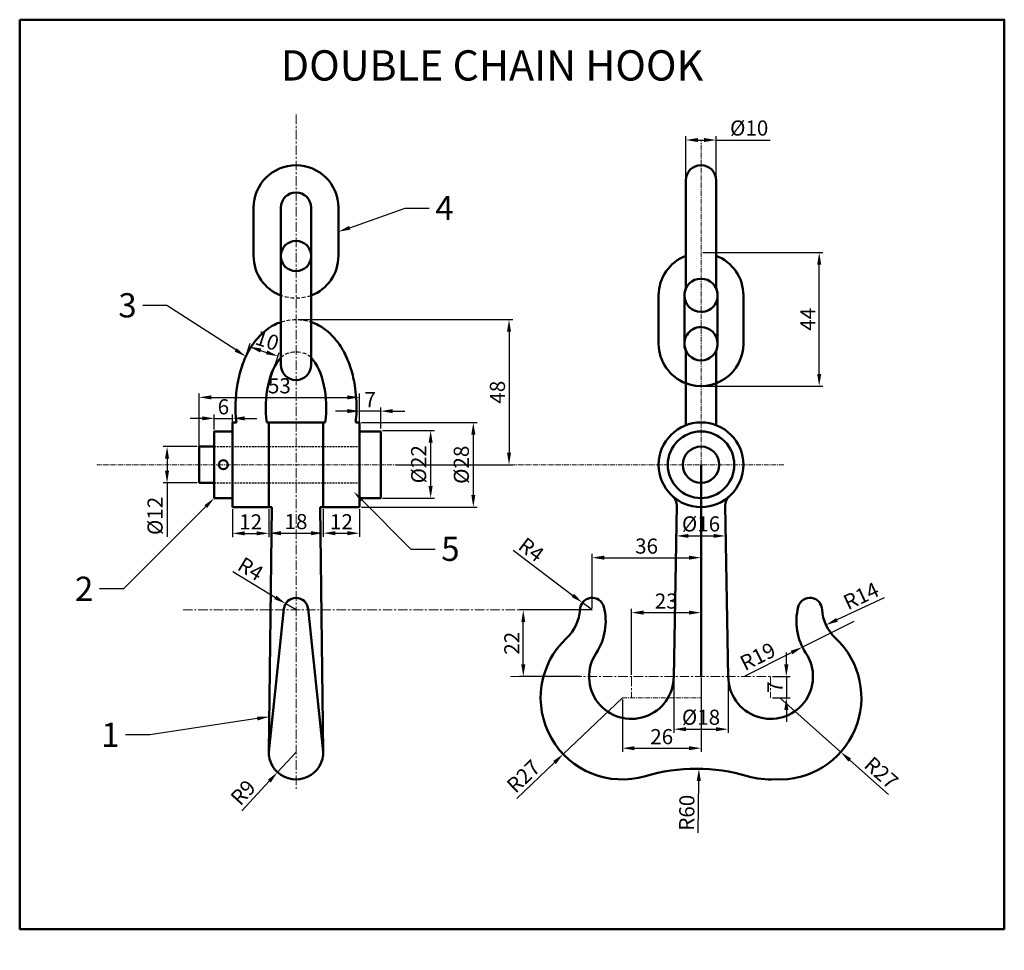
# Model space of a CAD drawing. Units: millimetres. Extents: x -60 to 265, y -36 to 271.
import ezdxf
from ezdxf import colors
from ezdxf.entities.mleader import LeaderData, LeaderLine
from ezdxf.math import Vec2, Vec3

# ---------------------------------------------------------------- set-up
doc = ezdxf.new("R2010")
doc.units = ezdxf.units.MM
doc.header["$LTSCALE"] = 0.1
doc.linetypes.add('CENTER', pattern=[50.8, 31.75, -6.35, 6.35, -6.35])
doc.linetypes.add('DASHED', pattern=[19.05, 12.7, -6.35])
for name, color, linetype, lineweight in [('M-CNTR', 1, 'CENTER', 18), ('M-DIMS', 2, 'Continuous', 25), ('M-HIDN', 4, 'DASHED', 25), ('M-OUTL', 7, 'Continuous', 50), ('M-TEXT', 3, 'Continuous', 25), ('M-TTLB', 7, 'Continuous', 50)]:
    doc.layers.add(name, color=color, linetype=linetype, lineweight=lineweight)
doc.styles.get("Standard").update_dxf_attribs({"font": 'arial.ttf'})
doc.dimstyles.new('ISO-25', dxfattribs={"dimtxt": 5, "dimasz": 4, "dimexe": 1.25, "dimexo": 0.625, "dimtad": 1, "dimdec": 0, "dimtxsty": 'Standard', "dimcen": 2.5, "dimadec": 0, "dimazin": 0, "dimtfac": 1, "dimtdec": 0, "dimtmove": 0, "dimatfit": 3, "dimfxl": 1, "dimarcsym": 0})

# ---------------------------------------------------------------- blocks, each defined once
blk = doc.blocks.new('*D1')
at = {"layer": 'Defpoints', "color": 0, "ltscale": 0.5, "transparency": 16777216}
for p in [(190.82, 47.23), (211, 29.28)]:
    blk.add_point(p, dxfattribs=at)
at = {"layer": 'M-DIMS', "color": 0, "lineweight": -2, "ltscale": 0.5, "transparency": 16777216}
for p, q in [((190.82, 47.23), (211, 29.28)), ((226.83, 15.2), (213.98, 26.63))]:
    blk.add_line(p, q, dxfattribs=at)
at = {"layer": 'M-DIMS', "color": 0, "ltscale": 0.5, "transparency": 16777216}
blk.add_solid([(214.43, 27.12), (213.54, 26.13), (211, 29.28)], dxfattribs=at)
at = {"layer": 'M-DIMS', "color": 0, "ltscale": 0.5, "transparency": 16777216, "insert": (223.99, 21.92), "char_height": 5, "attachment_point": 5, "rotation": 318.3453}
blk.add_mtext('R27', dxfattribs=at)
blk = doc.blocks.new('*D2')
at = {"layer": 'Defpoints', "color": 0, "ltscale": 0.5, "transparency": 16777216}
for p in [(164.12, 23.74), (163.32, -36.25)]:
    blk.add_point(p, dxfattribs=at)
at = {"layer": 'M-DIMS', "color": 0, "lineweight": -2, "ltscale": 0.5, "transparency": 16777216}
blk.add_line((163.84, 2.57), (164.07, 19.75), dxfattribs=at)
at = {"layer": 'M-DIMS', "color": 0, "ltscale": 0.5, "transparency": 16777216}
blk.add_solid([(163.4, 19.75), (164.74, 19.74), (164.12, 23.74)], dxfattribs=at)
at = {"layer": 'M-DIMS', "color": 0, "ltscale": 0.5, "transparency": 16777216, "insert": (160.75, 9.2), "char_height": 5, "attachment_point": 5, "rotation": 89.2359}
blk.add_mtext('R60', dxfattribs=at)
blk = doc.blocks.new('*D3')
at = {"layer": 'Defpoints', "color": 0, "ltscale": 0.5, "transparency": 16777216}
for p in [(218.8, 77.2), (206.11, 71.28)]:
    blk.add_point(p, dxfattribs=at)
at = {"layer": 'M-DIMS', "color": 0, "lineweight": -2, "ltscale": 0.5, "transparency": 16777216}
blk.add_line((225.3, 80.24), (209.74, 72.97), dxfattribs=at)
at = {"layer": 'M-DIMS', "color": 0, "ltscale": 0.5, "transparency": 16777216}
blk.add_solid([(209.45, 73.58), (210.02, 72.37), (206.11, 71.28)], dxfattribs=at)
at = {"layer": 'M-DIMS', "color": 0, "ltscale": 0.5, "transparency": 16777216, "insert": (218, 80.29), "char_height": 5, "attachment_point": 5, "rotation": 25.0408}
blk.add_mtext('R14', dxfattribs=at)
blk = doc.blocks.new('*D4')
at = {"layer": 'Defpoints', "color": 0, "ltscale": 0.5, "transparency": 16777216}
for p in [(215.34, 72.45), (198.33, 63.97)]:
    blk.add_point(p, dxfattribs=at)
at = {"layer": 'M-DIMS', "color": 0, "lineweight": -2, "ltscale": 0.5, "transparency": 16777216}
for p, q in [((215.34, 72.45), (198.33, 63.97)), ((179.36, 54.5), (194.76, 62.18))]:
    blk.add_line(p, q, dxfattribs=at)
at = {"layer": 'M-DIMS', "color": 0, "ltscale": 0.5, "transparency": 16777216}
blk.add_solid([(194.46, 62.78), (195.05, 61.59), (198.33, 63.97)], dxfattribs=at)
at = {"layer": 'M-DIMS', "color": 0, "ltscale": 0.5, "transparency": 16777216, "insert": (183.85, 60.3), "char_height": 5, "attachment_point": 5, "rotation": 26.5038}
blk.add_mtext('R19', dxfattribs=at)
blk = doc.blocks.new('*D5')
at = {"layer": 'Defpoints', "color": 0, "ltscale": 0.5, "transparency": 16777216}
for p in [(125.63, 78.64), (128.82, 76.23)]:
    blk.add_point(p, dxfattribs=at)
at = {"layer": 'M-DIMS', "color": 0, "lineweight": -2, "ltscale": 0.5, "transparency": 16777216}
for p, q in [((102.74, 95.97), (122.44, 81.06)), ((128.82, 76.23), (125.63, 78.64))]:
    blk.add_line(p, q, dxfattribs=at)
at = {"layer": 'M-DIMS', "color": 0, "ltscale": 0.5, "transparency": 16777216}
blk.add_solid([(122.85, 81.59), (122.04, 80.52), (125.63, 78.64)], dxfattribs=at)
at = {"layer": 'M-DIMS', "color": 0, "ltscale": 0.5, "transparency": 16777216, "insert": (108.33, 95.65), "char_height": 5, "attachment_point": 5, "rotation": 322.8841}
blk.add_mtext('R4', dxfattribs=at)
blk = doc.blocks.new('*D6')
at = {"layer": 'Defpoints', "color": 0, "ltscale": 0.5, "transparency": 16777216}
for p in [(164.82, 93.52), (128.82, 76.23), (164.82, 76.23)]:
    blk.add_point(p, dxfattribs=at)
at = {"layer": 'M-DIMS', "color": 0, "lineweight": -2, "ltscale": 0.5, "transparency": 16777216}
for p, q in [((128.82, 76.85), (128.82, 94.77)), ((164.82, 76.85), (164.82, 94.77)), ((132.82, 93.52), (160.82, 93.52))]:
    blk.add_line(p, q, dxfattribs=at)
at = {"layer": 'M-DIMS', "color": 0, "ltscale": 0.5, "transparency": 16777216}
for points in [[(132.82, 94.19), (132.82, 92.86), (128.82, 93.52)], [(160.82, 94.19), (160.82, 92.86), (164.82, 93.52)]]:
    blk.add_solid(points, dxfattribs=at)
at = {"layer": 'M-DIMS', "color": 0, "ltscale": 0.5, "transparency": 16777216, "insert": (146.82, 96.7), "char_height": 5, "attachment_point": 5}
blk.add_mtext('36', dxfattribs=at)
blk = doc.blocks.new('*D7')
at = {"layer": 'Defpoints', "color": 0, "ltscale": 0.5, "transparency": 16777216}
for p in [(106.08, 76.23), (128.82, 76.23), (125.49, 54.23)]:
    blk.add_point(p, dxfattribs=at)
at = {"layer": 'M-DIMS', "color": 0, "lineweight": -2, "ltscale": 0.5, "transparency": 16777216}
for p, q in [((128.2, 76.23), (104.83, 76.23)), ((106.08, 58.23), (106.08, 72.23)), ((124.87, 54.23), (104.83, 54.23))]:
    blk.add_line(p, q, dxfattribs=at)
at = {"layer": 'M-DIMS', "color": 0, "ltscale": 0.5, "transparency": 16777216}
for points in [[(105.41, 72.23), (106.74, 72.23), (106.08, 76.23)], [(105.41, 58.23), (106.74, 58.23), (106.08, 54.23)]]:
    blk.add_solid(points, dxfattribs=at)
at = {"layer": 'M-DIMS', "color": 0, "ltscale": 0.5, "transparency": 16777216, "insert": (102.94, 65.23), "char_height": 5, "attachment_point": 5, "rotation": 90}
blk.add_mtext('22', dxfattribs=at)
blk = doc.blocks.new('*D8')
at = {"layer": 'Defpoints', "color": 0, "ltscale": 0.5, "transparency": 16777216}
for p in [(164.82, 75.36), (141.82, 54.23), (164.82, 54.23)]:
    blk.add_point(p, dxfattribs=at)
at = {"layer": 'M-DIMS', "color": 0, "lineweight": -2, "ltscale": 0.5, "transparency": 16777216}
for p, q in [((141.82, 54.85), (141.82, 76.61)), ((145.82, 75.36), (160.82, 75.36)), ((164.82, 54.85), (164.82, 76.61))]:
    blk.add_line(p, q, dxfattribs=at)
at = {"layer": 'M-DIMS', "color": 0, "ltscale": 0.5, "transparency": 16777216}
for points in [[(145.82, 76.03), (145.82, 74.69), (141.82, 75.36)], [(160.82, 76.03), (160.82, 74.69), (164.82, 75.36)]]:
    blk.add_solid(points, dxfattribs=at)
at = {"layer": 'M-DIMS', "color": 0, "ltscale": 0.5, "transparency": 16777216, "insert": (153.32, 78.54), "char_height": 5, "attachment_point": 5}
blk.add_mtext('23', dxfattribs=at)
blk = doc.blocks.new('*D9')
at = {"layer": 'Defpoints', "color": 0, "ltscale": 0.5, "transparency": 16777216}
for p in [(155.82, 53.98), (173.82, 53.98), (173.82, 36.83)]:
    blk.add_point(p, dxfattribs=at)
at = {"layer": 'M-DIMS', "color": 0, "lineweight": -2, "ltscale": 0.5, "transparency": 16777216}
for p, q in [((155.82, 53.35), (155.82, 35.58)), ((173.82, 53.35), (173.82, 35.58)), ((159.82, 36.83), (169.82, 36.83))]:
    blk.add_line(p, q, dxfattribs=at)
at = {"layer": 'M-DIMS', "color": 0, "ltscale": 0.5, "transparency": 16777216}
for points in [[(159.82, 37.49), (159.82, 36.16), (155.82, 36.83)], [(169.82, 37.49), (169.82, 36.16), (173.82, 36.83)]]:
    blk.add_solid(points, dxfattribs=at)
at = {"layer": 'M-DIMS', "color": 0, "ltscale": 0.5, "transparency": 16777216, "insert": (164.82, 40.14), "char_height": 5, "attachment_point": 5}
blk.add_mtext('%%C18', dxfattribs=at)
blk = doc.blocks.new('*D10')
at = {"layer": 'Defpoints', "color": 0, "ltscale": 0.5, "transparency": 16777216}
for p in [(164.82, 54.51), (138.82, 47.23), (164.82, 30.55)]:
    blk.add_point(p, dxfattribs=at)
at = {"layer": 'M-DIMS', "color": 0, "lineweight": -2, "ltscale": 0.5, "transparency": 16777216}
for p, q in [((164.82, 53.88), (164.82, 29.3)), ((138.82, 46.6), (138.82, 29.3)), ((142.82, 30.55), (160.82, 30.55))]:
    blk.add_line(p, q, dxfattribs=at)
at = {"layer": 'M-DIMS', "color": 0, "ltscale": 0.5, "transparency": 16777216}
for points in [[(142.82, 31.22), (142.82, 29.88), (138.82, 30.55)], [(160.82, 31.22), (160.82, 29.88), (164.82, 30.55)]]:
    blk.add_solid(points, dxfattribs=at)
at = {"layer": 'M-DIMS', "color": 0, "ltscale": 0.5, "transparency": 16777216, "insert": (151.82, 33.73), "char_height": 5, "attachment_point": 5}
blk.add_mtext('26', dxfattribs=at)
blk = doc.blocks.new('*D11')
at = {"layer": 'Defpoints', "color": 0, "ltscale": 0.5, "transparency": 16777216}
for p in [(138.82, 47.23), (119.29, 28.59)]:
    blk.add_point(p, dxfattribs=at)
at = {"layer": 'M-DIMS', "color": 0, "lineweight": -2, "ltscale": 0.5, "transparency": 16777216}
for p, q in [((138.82, 47.23), (119.29, 28.59)), ((103.96, 13.95), (116.4, 25.83))]:
    blk.add_line(p, q, dxfattribs=at)
at = {"layer": 'M-DIMS', "color": 0, "ltscale": 0.5, "transparency": 16777216}
blk.add_solid([(115.94, 26.31), (116.86, 25.34), (119.29, 28.59)], dxfattribs=at)
at = {"layer": 'M-DIMS', "color": 0, "ltscale": 0.5, "transparency": 16777216, "insert": (106.57, 20.78), "char_height": 5, "attachment_point": 5, "rotation": 43.664}
blk.add_mtext('R27', dxfattribs=at)
blk = doc.blocks.new('*D12')
at = {"layer": 'Defpoints', "color": 0, "ltscale": 0.5, "transparency": 16777216}
for p in [(187.82, 54.23), (187.82, 47.23), (193.02, 47.23)]:
    blk.add_point(p, dxfattribs=at)
at = {"layer": 'M-DIMS', "color": 0, "lineweight": -2, "ltscale": 0.5, "transparency": 16777216}
for p, q in [((193.02, 58.23), (193.02, 62.23)), ((188.45, 54.23), (194.27, 54.23)), ((193.02, 54.23), (193.02, 47.23)), ((188.45, 47.23), (194.27, 47.23)), ((193.02, 43.23), (193.02, 39.23))]:
    blk.add_line(p, q, dxfattribs=at)
at = {"layer": 'M-DIMS', "color": 0, "ltscale": 0.5, "transparency": 16777216}
for points in [[(192.35, 58.23), (193.69, 58.23), (193.02, 54.23)], [(192.35, 43.23), (193.69, 43.23), (193.02, 47.23)]]:
    blk.add_solid(points, dxfattribs=at)
at = {"layer": 'M-DIMS', "color": 0, "ltscale": 0.5, "transparency": 16777216, "insert": (189.9, 50.73), "char_height": 5, "attachment_point": 5, "rotation": 90}
blk.add_mtext('7', dxfattribs=at)
blk = doc.blocks.new('*D13')
at = {"layer": 'Defpoints', "color": 0, "ltscale": 0.5, "transparency": 16777216}
for p in [(156.68, 102.06), (172.96, 102.35), (172.96, 100.71)]:
    blk.add_point(p, dxfattribs=at)
at = {"layer": 'M-DIMS', "color": 0, "lineweight": -2, "ltscale": 0.5, "transparency": 16777216}
for p, q in [((156.68, 101.43), (156.68, 99.46)), ((172.96, 101.72), (172.96, 99.46)), ((160.68, 100.71), (168.96, 100.71))]:
    blk.add_line(p, q, dxfattribs=at)
at = {"layer": 'M-DIMS', "color": 0, "ltscale": 0.5, "transparency": 16777216}
for points in [[(160.68, 101.38), (160.68, 100.05), (156.68, 100.71)], [(168.96, 101.38), (168.96, 100.05), (172.96, 100.71)]]:
    blk.add_solid(points, dxfattribs=at)
at = {"layer": 'M-DIMS', "color": 0, "ltscale": 0.5, "transparency": 16777216, "insert": (164.82, 104.03), "char_height": 5, "attachment_point": 5}
blk.add_mtext('%%C16', dxfattribs=at)
blk = doc.blocks.new('*U14')
at = {"layer": 'M-CNTR', "color": 0, "transparency": 16777216}
blk.add_line((0, 60.73), (0, -162.53), dxfattribs=at)
blk = doc.blocks.new('*D15')
at = {"layer": 'Defpoints', "color": 0, "ltscale": 0.1, "transparency": 16777216}
for p in [(51.96, 141.96), (51.96, 135.55), (58.96, 135.55)]:
    blk.add_point(p, dxfattribs=at)
at = {"layer": 'M-DIMS', "color": 0, "lineweight": -2, "ltscale": 0.1, "transparency": 16777216}
for p, q in [((51.96, 136.17), (51.96, 143.21)), ((58.96, 136.17), (58.96, 143.21)), ((47.96, 141.96), (43.96, 141.96)), ((58.96, 141.96), (51.96, 141.96)), ((62.96, 141.96), (66.96, 141.96))]:
    blk.add_line(p, q, dxfattribs=at)
at = {"layer": 'M-DIMS', "color": 0, "ltscale": 0.1, "transparency": 16777216}
for points in [[(47.96, 142.63), (47.96, 141.3), (51.96, 141.96)], [(62.96, 142.63), (62.96, 141.3), (58.96, 141.96)]]:
    blk.add_solid(points, dxfattribs=at)
at = {"layer": 'M-DIMS', "color": 0, "ltscale": 0.1, "transparency": 16777216, "insert": (55.46, 145.09), "char_height": 5, "attachment_point": 5}
blk.add_mtext('7', dxfattribs=at)
blk = doc.blocks.new('*D16')
at = {"layer": 'Defpoints', "color": 0, "ltscale": 0.1, "transparency": 16777216}
for p in [(9.96, 139.56), (3.96, 135.23), (9.96, 135.23)]:
    blk.add_point(p, dxfattribs=at)
at = {"layer": 'M-DIMS', "color": 0, "lineweight": -2, "ltscale": 0.1, "transparency": 16777216}
for p, q in [((3.96, 135.85), (3.96, 140.81)), ((9.96, 135.85), (9.96, 140.81)), ((-0.04, 139.56), (-4.04, 139.56)), ((3.96, 139.56), (9.96, 139.56)), ((13.96, 139.56), (17.96, 139.56))]:
    blk.add_line(p, q, dxfattribs=at)
at = {"layer": 'M-DIMS', "color": 0, "ltscale": 0.1, "transparency": 16777216}
for points in [[(-0.04, 140.23), (-0.04, 138.9), (3.96, 139.56)], [(13.96, 140.23), (13.96, 138.9), (9.96, 139.56)]]:
    blk.add_solid(points, dxfattribs=at)
at = {"layer": 'M-DIMS', "color": 0, "ltscale": 0.1, "transparency": 16777216, "insert": (6.96, 142.74), "char_height": 5, "attachment_point": 5}
blk.add_mtext('6', dxfattribs=at)
blk = doc.blocks.new('*D17')
at = {"layer": 'Defpoints', "color": 0, "ltscale": 0.1, "transparency": 16777216}
for p in [(51.96, 146.5), (-1.04, 124.23), (51.96, 124.23)]:
    blk.add_point(p, dxfattribs=at)
at = {"layer": 'M-DIMS', "color": 0, "lineweight": -2, "ltscale": 0.1, "transparency": 16777216}
for p, q in [((-1.04, 124.85), (-1.04, 147.75)), ((2.96, 146.5), (47.96, 146.5)), ((51.96, 124.85), (51.96, 147.75))]:
    blk.add_line(p, q, dxfattribs=at)
at = {"layer": 'M-DIMS', "color": 0, "ltscale": 0.1, "transparency": 16777216}
for points in [[(2.96, 147.17), (2.96, 145.84), (-1.04, 146.5)], [(47.96, 147.17), (47.96, 145.84), (51.96, 146.5)]]:
    blk.add_solid(points, dxfattribs=at)
at = {"layer": 'M-DIMS', "color": 0, "ltscale": 0.1, "transparency": 16777216, "insert": (25.46, 149.68), "char_height": 5, "attachment_point": 5}
blk.add_mtext('53', dxfattribs=at)
blk = doc.blocks.new('*D18')
at = {"layer": 'Defpoints', "color": 0, "ltscale": 0.1, "transparency": 16777216}
for p in [(-1.04, 130.23), (-11.66, 118.23), (-1.04, 118.23)]:
    blk.add_point(p, dxfattribs=at)
at = {"layer": 'M-DIMS', "color": 0, "lineweight": -2, "ltscale": 0.1, "transparency": 16777216}
for p, q in [((-1.66, 130.23), (-12.91, 130.23)), ((-11.66, 126.23), (-11.66, 122.23)), ((-1.66, 118.23), (-12.91, 118.23)), ((-11.66, 118.23), (-11.66, 100.43))]:
    blk.add_line(p, q, dxfattribs=at)
at = {"layer": 'M-DIMS', "color": 0, "ltscale": 0.1, "transparency": 16777216}
for points in [[(-12.33, 126.23), (-11, 126.23), (-11.66, 130.23)], [(-12.33, 122.23), (-11, 122.23), (-11.66, 118.23)]]:
    blk.add_solid(points, dxfattribs=at)
at = {"layer": 'M-DIMS', "color": 0, "ltscale": 0.1, "transparency": 16777216, "insert": (-14.98, 107.33), "char_height": 5, "attachment_point": 5, "rotation": 90}
blk.add_mtext('%%C12', dxfattribs=at)
blk = doc.blocks.new('*D19')
at = {"layer": 'Defpoints', "color": 0, "ltscale": 0.1, "transparency": 16777216}
for p in [(58.96, 135.55), (58.96, 113.23), (75.46, 113.23)]:
    blk.add_point(p, dxfattribs=at)
at = {"layer": 'M-DIMS', "color": 0, "lineweight": -2, "ltscale": 0.1, "transparency": 16777216}
for p, q in [((59.59, 135.55), (76.71, 135.55)), ((75.46, 131.55), (75.46, 117.23)), ((59.59, 113.23), (76.71, 113.23))]:
    blk.add_line(p, q, dxfattribs=at)
at = {"layer": 'M-DIMS', "color": 0, "ltscale": 0.1, "transparency": 16777216}
for points in [[(74.79, 131.55), (76.13, 131.55), (75.46, 135.55)], [(74.79, 117.23), (76.13, 117.23), (75.46, 113.23)]]:
    blk.add_solid(points, dxfattribs=at)
at = {"layer": 'M-DIMS', "color": 0, "ltscale": 0.1, "transparency": 16777216, "insert": (72.14, 124.39), "char_height": 5, "attachment_point": 5, "rotation": 90}
blk.add_mtext('%%C22', dxfattribs=at)
blk = doc.blocks.new('*D20')
at = {"layer": 'Defpoints', "color": 0, "ltscale": 0.1, "transparency": 16777216}
for p in [(51.96, 138.23), (51.96, 110.23), (89.56, 110.23)]:
    blk.add_point(p, dxfattribs=at)
at = {"layer": 'M-DIMS', "color": 0, "lineweight": -2, "ltscale": 0.1, "transparency": 16777216}
for p, q in [((52.59, 138.23), (90.81, 138.23)), ((89.56, 134.23), (89.56, 114.23)), ((52.59, 110.23), (90.81, 110.23))]:
    blk.add_line(p, q, dxfattribs=at)
at = {"layer": 'M-DIMS', "color": 0, "ltscale": 0.1, "transparency": 16777216}
for points in [[(88.9, 134.23), (90.23, 134.23), (89.56, 138.23)], [(88.9, 114.23), (90.23, 114.23), (89.56, 110.23)]]:
    blk.add_solid(points, dxfattribs=at)
at = {"layer": 'M-DIMS', "color": 0, "ltscale": 0.1, "transparency": 16777216, "insert": (86.25, 124.23), "char_height": 5, "attachment_point": 5, "rotation": 90}
blk.add_mtext('%%C28', dxfattribs=at)
blk = doc.blocks.new('*D21')
at = {"layer": 'Defpoints', "color": 0, "ltscale": 0.1, "transparency": 16777216}
for p in [(9.96, 110.23), (21.96, 110.23), (21.96, 101.56)]:
    blk.add_point(p, dxfattribs=at)
at = {"layer": 'M-DIMS', "color": 0, "lineweight": -2, "ltscale": 0.1, "transparency": 16777216}
for p, q in [((9.96, 109.6), (9.96, 100.31)), ((21.96, 109.6), (21.96, 100.31)), ((13.96, 101.56), (17.96, 101.56))]:
    blk.add_line(p, q, dxfattribs=at)
at = {"layer": 'M-DIMS', "color": 0, "ltscale": 0.1, "transparency": 16777216}
for points in [[(13.96, 102.23), (13.96, 100.9), (9.96, 101.56)], [(17.96, 102.23), (17.96, 100.9), (21.96, 101.56)]]:
    blk.add_solid(points, dxfattribs=at)
at = {"layer": 'M-DIMS', "color": 0, "ltscale": 0.1, "transparency": 16777216, "insert": (15.96, 104.7), "char_height": 5, "attachment_point": 5}
blk.add_mtext('12', dxfattribs=at)
blk = doc.blocks.new('*D22')
at = {"layer": 'Defpoints', "color": 0, "ltscale": 0.1, "transparency": 16777216}
for p in [(21.96, 110.23), (39.96, 110.23), (39.96, 101.62)]:
    blk.add_point(p, dxfattribs=at)
at = {"layer": 'M-DIMS', "color": 0, "lineweight": -2, "ltscale": 0.1, "transparency": 16777216}
for p, q in [((21.96, 109.6), (21.96, 100.37)), ((39.96, 109.6), (39.96, 100.37)), ((25.96, 101.62), (35.96, 101.62))]:
    blk.add_line(p, q, dxfattribs=at)
at = {"layer": 'M-DIMS', "color": 0, "ltscale": 0.1, "transparency": 16777216}
for points in [[(25.96, 102.28), (25.96, 100.95), (21.96, 101.62)], [(35.96, 102.28), (35.96, 100.95), (39.96, 101.62)]]:
    blk.add_solid(points, dxfattribs=at)
at = {"layer": 'M-DIMS', "color": 0, "ltscale": 0.1, "transparency": 16777216, "insert": (30.96, 104.8), "char_height": 5, "attachment_point": 5}
blk.add_mtext('18', dxfattribs=at)
blk = doc.blocks.new('*D23')
at = {"layer": 'Defpoints', "color": 0, "ltscale": 0.1, "transparency": 16777216}
for p in [(39.96, 110.23), (51.96, 110.23), (51.96, 101.62)]:
    blk.add_point(p, dxfattribs=at)
at = {"layer": 'M-DIMS', "color": 0, "lineweight": -2, "ltscale": 0.1, "transparency": 16777216}
for p, q in [((39.96, 109.6), (39.96, 100.37)), ((51.96, 109.6), (51.96, 100.37)), ((43.96, 101.62), (47.96, 101.62))]:
    blk.add_line(p, q, dxfattribs=at)
at = {"layer": 'M-DIMS', "color": 0, "ltscale": 0.1, "transparency": 16777216}
for points in [[(43.96, 102.28), (43.96, 100.95), (39.96, 101.62)], [(47.96, 102.28), (47.96, 100.95), (51.96, 101.62)]]:
    blk.add_solid(points, dxfattribs=at)
at = {"layer": 'M-DIMS', "color": 0, "ltscale": 0.1, "transparency": 16777216, "insert": (45.96, 104.75), "char_height": 5, "attachment_point": 5}
blk.add_mtext('12', dxfattribs=at)
blk = doc.blocks.new('*D24')
at = {"layer": 'Defpoints', "color": 0, "ltscale": 0.1, "transparency": 16777216}
for p in [(27.55, 78.31), (30.96, 76.23)]:
    blk.add_point(p, dxfattribs=at)
at = {"layer": 'M-DIMS', "color": 0, "lineweight": -2, "ltscale": 0.1, "transparency": 16777216}
for p, q in [((10.03, 89), (24.13, 80.39)), ((30.96, 76.23), (27.55, 78.31))]:
    blk.add_line(p, q, dxfattribs=at)
at = {"layer": 'M-DIMS', "color": 0, "ltscale": 0.1, "transparency": 16777216}
blk.add_solid([(24.48, 80.96), (23.79, 79.83), (27.55, 78.31)], dxfattribs=at)
at = {"layer": 'M-DIMS', "color": 0, "ltscale": 0.1, "transparency": 16777216, "insert": (15.62, 89.25), "char_height": 5, "attachment_point": 5, "rotation": 328.6196}
blk.add_mtext('R4', dxfattribs=at)
blk = doc.blocks.new('*D25')
at = {"layer": 'Defpoints', "color": 0, "ltscale": 0.1, "transparency": 16777216}
for p in [(30.96, 29.23), (24.85, 22.62)]:
    blk.add_point(p, dxfattribs=at)
at = {"layer": 'M-DIMS', "color": 0, "lineweight": -2, "ltscale": 0.1, "transparency": 16777216}
for p, q in [((30.96, 29.23), (24.85, 22.62)), ((13.1, 9.9), (22.14, 19.68))]:
    blk.add_line(p, q, dxfattribs=at)
at = {"layer": 'M-DIMS', "color": 0, "ltscale": 0.1, "transparency": 16777216}
blk.add_solid([(21.65, 20.13), (22.63, 19.23), (24.85, 22.62)], dxfattribs=at)
at = {"layer": 'M-DIMS', "color": 0, "ltscale": 0.1, "transparency": 16777216, "insert": (13.93, 15.48), "char_height": 5, "attachment_point": 5, "rotation": 47.2558}
blk.add_mtext('R9', dxfattribs=at)
blk = doc.blocks.new('*D26')
at = {"layer": 'Defpoints', "color": 0, "ltscale": 0.1, "transparency": 16777216}
for p in [(164.82, 194.38), (203.87, 194.38), (164.82, 150.23)]:
    blk.add_point(p, dxfattribs=at)
at = {"layer": 'M-DIMS', "color": 0, "lineweight": -2, "ltscale": 0.1, "transparency": 16777216}
for p, q in [((165.45, 194.38), (205.12, 194.38)), ((203.87, 154.23), (203.87, 190.38)), ((165.45, 150.23), (205.12, 150.23))]:
    blk.add_line(p, q, dxfattribs=at)
at = {"layer": 'M-DIMS', "color": 0, "ltscale": 0.1, "transparency": 16777216}
for points in [[(203.21, 190.38), (204.54, 190.38), (203.87, 194.38)], [(203.21, 154.23), (204.54, 154.23), (203.87, 150.23)]]:
    blk.add_solid(points, dxfattribs=at)
at = {"layer": 'M-DIMS', "color": 0, "ltscale": 0.1, "transparency": 16777216, "insert": (200.75, 172.31), "char_height": 5, "attachment_point": 5, "rotation": 90}
blk.add_mtext('44', dxfattribs=at)
blk = doc.blocks.new('*D27')
at = {"layer": 'Defpoints', "color": 0, "ltscale": 0.1, "transparency": 16777216}
for p in [(169.82, 231.56), (159.82, 210.23), (169.82, 210.23)]:
    blk.add_point(p, dxfattribs=at)
at = {"layer": 'M-DIMS', "color": 0, "lineweight": -2, "ltscale": 0.1, "transparency": 16777216}
for p, q in [((159.82, 210.85), (159.82, 232.81)), ((163.82, 231.56), (165.82, 231.56)), ((169.82, 210.85), (169.82, 232.81)), ((169.82, 231.56), (187.66, 231.56))]:
    blk.add_line(p, q, dxfattribs=at)
at = {"layer": 'M-DIMS', "color": 0, "ltscale": 0.1, "transparency": 16777216}
for points in [[(163.82, 232.23), (163.82, 230.89), (159.82, 231.56)], [(165.82, 232.23), (165.82, 230.89), (169.82, 231.56)]]:
    blk.add_solid(points, dxfattribs=at)
at = {"layer": 'M-DIMS', "color": 0, "ltscale": 0.1, "transparency": 16777216, "insert": (180.74, 234.88), "char_height": 5, "attachment_point": 5}
blk.add_mtext('%%C10', dxfattribs=at)
blk = doc.blocks.new('*D28')
at = {"layer": 'Defpoints', "color": 0, "ltscale": 0.1, "transparency": 16777216}
for p in [(30.96, 172.2), (63.39, 124.23), (101.36, 124.23)]:
    blk.add_point(p, dxfattribs=at)
at = {"layer": 'M-DIMS', "color": 0, "lineweight": -2, "ltscale": 0.1, "transparency": 16777216}
for p, q in [((31.59, 172.2), (102.61, 172.2)), ((101.36, 168.2), (101.36, 128.23)), ((64.01, 124.23), (102.61, 124.23))]:
    blk.add_line(p, q, dxfattribs=at)
at = {"layer": 'M-DIMS', "color": 0, "ltscale": 0.1, "transparency": 16777216}
for points in [[(100.69, 168.2), (102.03, 168.2), (101.36, 172.2)], [(100.69, 128.23), (102.03, 128.23), (101.36, 124.23)]]:
    blk.add_solid(points, dxfattribs=at)
at = {"layer": 'M-DIMS', "color": 0, "ltscale": 0.1, "transparency": 16777216, "insert": (98.18, 148.21), "char_height": 5, "attachment_point": 5, "rotation": 90}
blk.add_mtext('48', dxfattribs=at)
blk = doc.blocks.new('*D29')
at = {"layer": 'Defpoints', "color": 0, "ltscale": 0.1, "transparency": 16777216}
for p in [(25.04, 160.12), (11.95, 152.62), (21.52, 149.46)]:
    blk.add_point(p, dxfattribs=at)
at = {"layer": 'M-DIMS', "color": 0, "lineweight": -2, "ltscale": 0.1, "transparency": 16777216}
for p, q in [((12.15, 153.22), (15.86, 164.47)), ((19.27, 162.03), (21.24, 161.38)), ((21.71, 150.06), (25.43, 161.31))]:
    blk.add_line(p, q, dxfattribs=at)
at = {"layer": 'M-DIMS', "color": 0, "ltscale": 0.1, "transparency": 16777216}
for points in [[(19.48, 162.66), (19.06, 161.39), (15.47, 163.28)], [(21.45, 162.01), (21.03, 160.74), (25.04, 160.12)]]:
    blk.add_solid(points, dxfattribs=at)
at = {"layer": 'M-DIMS', "color": 0, "ltscale": 0.1, "transparency": 16777216, "insert": (21.25, 164.72), "char_height": 5, "attachment_point": 5, "rotation": 341.7212}
blk.add_mtext('10', dxfattribs=at)

msp = doc.modelspace()

# ---------------------------------------------------------------- linework, layer by layer
at = {"layer": 'M-CNTR', "ltscale": 0.5}
for p, q in [((164.82, 124.23), (164.82, 231.04)), ((192.24, 124.23), (-34.91, 124.23)), ((138.82, 47.23), (164.82, 47.23))]:
    msp.add_line(p, q, dxfattribs=at)
at = {"layer": 'M-CNTR'}
for p, q in [((128.82, 76.23), (-6.37, 76.23)), ((101.9, 54.23), (187.82, 54.23)), ((141.82, 54.23), (141.82, 47.23)), ((187.82, 54.23), (187.82, 47.23))]:
    msp.add_line(p, q, dxfattribs=at)
at = {"layer": 'M-HIDN', "ltscale": 0.5}
for p, q in [((3.96, 130.23), (51.96, 130.23)), ((3.96, 118.23), (51.96, 118.23))]:
    msp.add_line(p, q, dxfattribs=at)
at = {"layer": 'M-HIDN'}
for points in [[(35.96, 180.15), (32.85, 178.96), (29.08, 178.96), (25.96, 180.15)], [(25.96, 171.39), (29.12, 172.47), (32.81, 172.47), (35.96, 171.39)], [(25.96, 159.68), (28.21, 162.15), (33.72, 162.15), (35.96, 159.68)]]:
    msp.add_open_spline(points, degree=3, dxfattribs=at)
at = {"layer": 'M-OUTL', "ltscale": 0.5}
for p, q in [((159.82, 218.23), (159.82, 202.23)), ((25.96, 209.23), (25.96, 193.23)), ((9.96, 138.23), (9.96, 110.23)), ((9.96, 138.23), (10.96, 138.23)), ((10.96, 138.23), (11.24, 138.23)), ((21.31, 138.23), (21.96, 138.23)), ((40.61, 138.23), (21.96, 138.23)), ((21.96, 110.23), (21.96, 138.23)), ((39.96, 110.23), (39.96, 138.23)), ((51.96, 138.23), (50.69, 138.23)), ((51.96, 110.23), (51.96, 138.23)), ((51.96, 135.23), (58.96, 135.23)), ((58.96, 135.23), (58.96, 113.23)), ((-1.04, 118.23), (-1.04, 130.23)), ((-1.04, 130.23), (3.96, 130.23)), ((-1.04, 118.23), (3.96, 118.23)), ((58.96, 113.23), (51.96, 113.23)), ((9.96, 110.23), (22.96, 110.23)), ((22.96, 110.23), (21.96, 29.34)), ((38.96, 110.23), (39.96, 29.34)), ((38.96, 110.23), (51.96, 110.23)), ((26.98, 76.65), (21.96, 29.34)), ((34.94, 76.65), (39.96, 29.34))]:
    msp.add_line(p, q, dxfattribs=at)
at = {"layer": 'M-OUTL', "ltscale": 0.1}
for p, q in [((159.32, 180.23), (159.32, 164.23)), ((170.32, 180.23), (170.32, 164.23))]:
    msp.add_line(p, q, dxfattribs=at)
at = {"layer": 'M-OUTL'}
for p, q in [((164.82, 124.23), (164.82, 54.23)), ((156.83, 110.73), (155.82, 53.98)), ((172.81, 110.73), (173.82, 53.98))]:
    msp.add_line(p, q, dxfattribs=at)
at = {"layer": 'M-OUTL', "ltscale": 0.5}
for points in [[(35.96, 180.15, 0.310868), (44.96, 193.23), (44.96, 209.23, 1), (16.96, 209.23), (16.96, 193.23, 0.310868), (25.96, 180.15, 0.310868)], [(159.82, 218.23, -1), (169.82, 218.23), (169.82, 202.23)], [(25.96, 209.23, -1), (35.96, 209.23), (35.96, 193.23)], [(35.96, 201.23), (35.96, 157.23, -1), (25.96, 157.23), (25.96, 201.23)]]:
    msp.add_lwpolyline(points, format="xyb", dxfattribs=at)
for points in [[(159.82, 182.52), (159.82, 210.23)], [(169.82, 210.23), (169.82, 182.52)], [(159.82, 137.31), (159.82, 161.94)], [(169.82, 161.94), (169.82, 137.31)]]:
    msp.add_lwpolyline(points, dxfattribs=at)
at = {"layer": 'M-OUTL', "ltscale": 0.1}
for points in [[(159.82, 193.31, 0.310868), (150.82, 180.23), (150.82, 164.23, 0.310868), (159.82, 151.15)], [(159.82, 151.15, 0.525707), (178.82, 164.23), (178.82, 180.23, 0.310868), (169.82, 193.31, 0.310868)]]:
    msp.add_lwpolyline(points, format="xyb", dxfattribs=at)
at = {"layer": 'M-OUTL', "ltscale": 0.5}
msp.add_lwpolyline([(3.96, 113.23), (3.96, 135.23), (9.96, 135.23), (9.96, 113.23)], close=True, dxfattribs=at)
at = {"layer": 'M-OUTL', "ltscale": 0.1}
for centre, radius in [((30.96, 193.23), 5), ((6.96, 124.23), 1.5)]:
    msp.add_circle(centre, radius, dxfattribs=at)
at = {"layer": 'M-OUTL'}
for radius in [14, 11, 6]:
    msp.add_circle((164.82, 124.23), radius, dxfattribs=at)
at = {"layer": 'M-OUTL', "ltscale": 0.1}
for centre, start, end in [((164.82, 180.23), 0, 180), ((164.82, 180.23), 90, 270), ((164.82, 180.23), 155.38, 180), ((164.82, 180.23), 270, 24.62), ((164.82, 180.23), 0, 24.62), ((164.82, 164.23), 180, 90), ((164.82, 164.23), 90, 204.62), ((164.82, 164.23), 335.38, 0)]:
    msp.add_arc(centre, 5.5, start, end, dxfattribs=at)
at = {"layer": 'M-OUTL'}
for centre, radius, start, end in [((152.83, 110.8), 4, 358.9792, 48.2307), ((176.81, 110.8), 4, 131.7693, 181.0208), ((128.82, 76.23), 4, 14.6032, 180), ((200.82, 76.23), 4, 0, 165.3968), ((114.31, 72.45), 19, 326.4912, 14.6032), ((215.34, 72.45), 19, 165.3968, 213.5088), ((141.82, 54.23), 14, 146.4912, 0), ((187.82, 54.23), 14, 180, 33.5088), ((187.82, 47.23), 27, 253.6437, 273.1847)]:
    msp.add_arc(centre, radius, start, end, dxfattribs=at)
at = {"layer": 'M-OUTL', "ltscale": 0.5}
for centre, radius, start, end in [((30.96, 76.23), 4, 6.0588, 173.9412), ((110.85, 77.2), 14, 313.0223, 356.8962), ((218.8, 77.2), 14, 183.1038, 226.9777), ((138.82, 47.23), 27, 133.0223, 286.3563), ((190.82, 47.23), 27, 266.8153, 46.9777), ((138.82, 47.23), 27, 15.0261, 15.6425), ((30.96, 29.23), 9, 168.5903, 11.4097), ((163.32, -36.25), 60, 73.6437, 106.3563)]:
    msp.add_arc(centre, radius, start, end, dxfattribs=at)
for start_param, end_param in [(9.948377, 11.261868), (7.587688, 8.901179)]:
    msp.add_ellipse((30.96, 143.23), major_axis=(0, -19), ratio=0.526316, start_param=start_param, end_param=end_param, dxfattribs=at)
for points, knots in [([(25.96, 171.39), (25.23, 171.14), (24.53, 170.85), (22.87, 170), (21.95, 169.41), (20.27, 168.12), (19.5, 167.41), (18.11, 165.94), (17.49, 165.16), (15.73, 162.71), (14.78, 160.95), (13.2, 157.26), (12.59, 155.34), (11.65, 151.37), (11.32, 149.34), (10.96, 145.22), (10.92, 143.13), (11.06, 140.12), (11.13, 139.17), (11.24, 138.23)], [9.602601, 9.602601, 9.602601, 9.602601, 9.685359, 9.685359, 9.809715, 9.809715, 9.93407, 9.93407, 10.058426, 10.058426, 10.31504, 10.31504, 10.571653, 10.571653, 10.828267, 10.828267, 11.084881, 11.084881, 11.202425, 11.202425, 11.202425, 11.202425]), ([(50.69, 138.23), (50.82, 139.44), (50.91, 140.67), (51.03, 144.77), (50.84, 147.66), (50.02, 152.71), (49.48, 154.9), (48.14, 158.74), (47.41, 160.4), (45.78, 163.31), (44.92, 164.58), (43.08, 166.77), (42.15, 167.7), (40.01, 169.41), (38.81, 170.18), (36.99, 171.01), (36.48, 171.22), (35.96, 171.39)], [7.64713, 7.64713, 7.64713, 7.64713, 7.798841, 7.798841, 8.154578, 8.154578, 8.438847, 8.438847, 8.671929, 8.671929, 8.865707, 8.865707, 9.026822, 9.026822, 9.187937, 9.187937, 9.246951, 9.246951, 9.246951, 9.246951])]:
    msp.add_open_spline(points, degree=3, knots=knots, dxfattribs=at)
at = {"layer": 'M-TTLB', "ltscale": 0.1}
msp.add_lwpolyline([(-60.37, 271.33), (265.06, 271.33), (265.06, -29.25), (-60.37, -29.25)], close=True, dxfattribs=at)

# ---------------------------------------------------------------- block references
at = {"layer": 'M-CNTR'}
msp.add_blockref('*U14', (30.96, 179.23), dxfattribs=at)

# ---------------------------------------------------------------- texts
at = {"layer": 'M-TEXT', "ltscale": 0.1, "insert": (25.91, 261.22), "char_height": 10, "attachment_point": 1}
msp.add_mtext_dynamic_manual_height_columns('DOUBLE CHAIN HOOK', width=186.9101, gutter_width=12.5, heights=[0], dxfattribs=at)

# ---------------------------------------------------------------- dimensions: what is measured, and where the dimension line sits
at = {"layer": 'M-DIMS', "ltscale": 0.1}
dim = msp.add_linear_dim(base=(169.82, 231.56), p1=(159.82, 210.23), p2=(169.82, 210.23), text='%%C<>', dimstyle='ISO-25', override={"dimclrd": 0, "dimclre": 0, "dimclrt": 0}, dxfattribs=at)
dim.commit()
dim.dimension.update_dxf_attribs({"geometry": '*D27', "text_midpoint": (180.74, 234.88)})
for base, p1, p2, picture, middle in [((203.87, 194.38), (164.82, 150.23), (164.82, 194.38), '*D26', (200.75, 172.31)), ((101.36, 124.23), (30.96, 172.2), (63.39, 124.23), '*D28', (98.18, 148.21))]:
    dim = msp.add_linear_dim(base=base, p1=p1, p2=p2, angle=90, dimstyle='ISO-25', override={"dimclrd": 0, "dimclre": 0, "dimclrt": 0}, dxfattribs=at)
    dim.commit()
    dim.dimension.update_dxf_attribs({"geometry": picture, "text_midpoint": middle})
dim = msp.add_aligned_dim(p1=(11.95, 152.62), p2=(21.52, 149.46), distance=11.23, dimstyle='ISO-25', override={"dimclrd": 0, "dimclre": 0, "dimclrt": 0}, dxfattribs=at)
dim.commit()
dim.dimension.update_dxf_attribs({"geometry": '*D29', "text_midpoint": (21.25, 164.72)})
for base, p1, p2, picture, middle in [((51.96, 146.5), (-1.04, 124.23), (51.96, 124.23), '*D17', (25.46, 149.68)), ((51.96, 141.96), (58.96, 135.55), (51.96, 135.55), '*D15', (55.46, 145.09)), ((39.96, 101.62), (21.96, 110.23), (39.96, 110.23), '*D22', (30.96, 104.8)), ((51.96, 101.62), (39.96, 110.23), (51.96, 110.23), '*D23', (45.96, 104.75))]:
    dim = msp.add_linear_dim(base=base, p1=p1, p2=p2, dimstyle='ISO-25', override={"dimclrd": 0, "dimclre": 0, "dimclrt": 0}, dxfattribs=at)
    dim.commit()
    dim.dimension.update_dxf_attribs({"geometry": picture, "text_midpoint": middle})
for base, p1, p2, picture, middle in [((9.96, 139.56), (3.96, 135.23), (9.96, 135.23), '*D16', (6.96, 139.56)), ((21.96, 101.56), (9.96, 110.23), (21.96, 110.23), '*D21', (15.96, 101.56))]:
    dim = msp.add_linear_dim(base=base, p1=p1, p2=p2, dimstyle='ISO-25', override={"dimclrd": 0, "dimclre": 0, "dimclrt": 0}, dxfattribs=at)
    dim.commit()
    dim.dimension.update_dxf_attribs({"geometry": picture, "text_midpoint": middle, "dimtype": 160})
for base, p1, p2, picture, middle in [((89.56, 110.23), (51.96, 138.23), (51.96, 110.23), '*D20', (86.25, 124.23)), ((75.46, 113.23), (58.96, 135.55), (58.96, 113.23), '*D19', (72.14, 124.39)), ((-11.66, 118.23), (-1.04, 130.23), (-1.04, 118.23), '*D18', (-14.98, 107.33))]:
    dim = msp.add_linear_dim(base=base, p1=p1, p2=p2, angle=90, text='%%C<>', dimstyle='ISO-25', override={"dimclrd": 0, "dimclre": 0, "dimclrt": 0}, dxfattribs=at)
    dim.commit()
    dim.dimension.update_dxf_attribs({"geometry": picture, "text_midpoint": middle})
at = {"layer": 'M-DIMS', "ltscale": 0.5}
for base, p1, p2, picture, middle in [((172.96, 100.71), (156.68, 102.06), (172.96, 102.35), '*D13', (164.82, 104.03)), ((173.82, 36.83), (155.82, 53.98), (173.82, 53.98), '*D9', (164.82, 40.14))]:
    dim = msp.add_linear_dim(base=base, p1=p1, p2=p2, text='%%C<>', dimstyle='ISO-25', override={"dimclrd": 0, "dimclre": 0, "dimclrt": 0}, dxfattribs=at)
    dim.commit()
    dim.dimension.update_dxf_attribs({"geometry": picture, "text_midpoint": middle})
for center, mpoint, picture, middle in [((128.82, 76.23), (125.63, 78.64), '*D5', (106.45, 93.16)), ((218.8, 77.2), (206.11, 71.28), '*D3', (219.33, 77.45)), ((163.32, -36.25), (164.12, 23.74), '*D2', (163.93, 9.16))]:
    dim = msp.add_radius_dim(center=center, mpoint=mpoint, dimstyle='ISO-25', override={"dimclrd": 0, "dimclre": 0, "dimclrt": 0}, dxfattribs=at)
    dim.commit()
    dim.dimension.update_dxf_attribs({"geometry": picture, "text_midpoint": middle, "dimtype": 164})
for base, p1, p2, picture, middle in [((164.82, 93.52), (128.82, 76.23), (164.82, 76.23), '*D6', (146.82, 96.7)), ((164.82, 75.36), (141.82, 54.23), (164.82, 54.23), '*D8', (153.32, 78.54)), ((164.82, 30.55), (138.82, 47.23), (164.82, 54.51), '*D10', (151.82, 33.73))]:
    dim = msp.add_linear_dim(base=base, p1=p1, p2=p2, dimstyle='ISO-25', override={"dimclrd": 0, "dimclre": 0, "dimclrt": 0}, dxfattribs=at)
    dim.commit()
    dim.dimension.update_dxf_attribs({"geometry": picture, "text_midpoint": middle})
at = {"layer": 'M-DIMS', "ltscale": 0.1}
dim = msp.add_radius_dim(center=(30.96, 76.23), mpoint=(27.55, 78.31), dimstyle='ISO-25', override={"dimclrd": 0, "dimclre": 0, "dimclrt": 0}, dxfattribs=at)
dim.commit()
dim.dimension.update_dxf_attribs({"geometry": '*D24', "text_midpoint": (13.99, 86.58), "dimtype": 164})
at = {"layer": 'M-DIMS', "ltscale": 0.5}
for base, p1, p2, picture, middle in [((106.08, 76.23), (125.49, 54.23), (128.82, 76.23), '*D7', (102.94, 65.23)), ((193.02, 47.23), (187.82, 54.23), (187.82, 47.23), '*D12', (189.9, 50.73))]:
    dim = msp.add_linear_dim(base=base, p1=p1, p2=p2, angle=90, dimstyle='ISO-25', override={"dimclrd": 0, "dimclre": 0, "dimclrt": 0}, dxfattribs=at)
    dim.commit()
    dim.dimension.update_dxf_attribs({"geometry": picture, "text_midpoint": middle})
for center, mpoint, picture, middle in [((215.34, 72.45), (198.33, 63.97), '*D4', (183.85, 60.3)), ((138.82, 47.23), (119.29, 28.59), '*D11', (106.57, 20.78)), ((190.82, 47.23), (211, 29.28), '*D1', (223.99, 21.92))]:
    dim = msp.add_radius_dim(center=center, mpoint=mpoint, dimstyle='ISO-25', override={"dimclrd": 0, "dimclre": 0, "dimclrt": 0}, dxfattribs=at)
    dim.commit()
    dim.dimension.update_dxf_attribs({"geometry": picture, "text_midpoint": middle})
at = {"layer": 'M-DIMS', "ltscale": 0.1}
dim = msp.add_radius_dim(center=(30.96, 29.23), mpoint=(24.85, 22.62), dimstyle='ISO-25', override={"dimclrd": 0, "dimclre": 0, "dimclrt": 0}, dxfattribs=at)
dim.commit()
dim.dimension.update_dxf_attribs({"geometry": '*D25', "text_midpoint": (13.93, 15.48)})

# ---------------------------------------------------------------- leaders
at = {"layer": 'M-TEXT', "ltscale": 0.1}
ml = msp.add_multileader_mtext('Standard', dxfattribs=at)
ml.set_content('4', color=256)
ml.set_leader_properties()
ml.build(insert=Vec2(0, 0))
ctx = ml.context
ctx.base_point, ctx.char_height, ctx.plane_origin = Vec3(74.99, 209.09), 8, Vec3(44.96, 201.23)
notes = []
notes.append((ctx, [(0, (1, 1, 0), (66.99, 209.09), (1, 0), 8, [(0, [(44.96, 201.23)], 0, [])])]))
ctx.mtext.insert, ctx.mtext.flow_direction = Vec3(76.99, 213.09), 5
ml = msp.add_multileader_mtext('Standard', dxfattribs=at)
ml.set_content('3', color=256)
ml.set_leader_properties()
ml.build(insert=Vec2(0, 0))
ctx = ml.context
ctx.base_point, ctx.char_height, ctx.plane_origin = Vec3(-28.94, 176.86), 8, Vec3(14.39, 160.01)
ctx.text_align_type = 2
notes.append((ctx, [(0, (1, 1, 0), (-11.7, 176.86), (-1, 0), 8, [(0, [(14.39, 160.01)], 0, [])])]))
ctx.mtext.insert, ctx.mtext.alignment, ctx.mtext.flow_direction = Vec3(-21.7, 180.93), 3, 5
ml = msp.add_multileader_mtext('Standard', dxfattribs=at)
ml.set_content('5', color=256)
ml.set_leader_properties()
ml.build(insert=Vec2(0, 0))
ctx = ml.context
ctx.base_point, ctx.char_height, ctx.plane_origin = Vec3(76.96, 96.38), 8, Vec3(49.99, 115.35)
notes.append((ctx, [(0, (1, 1, 0), (68.96, 96.38), (1, 0), 8, [(0, [(49.99, 115.35)], 0, [])])]))
ctx.mtext.insert, ctx.mtext.flow_direction = Vec3(78.96, 100.45), 5
ml = msp.add_multileader_mtext('Standard', dxfattribs=at)
ml.set_content('2', color=256)
ml.set_leader_properties()
ml.build(insert=Vec2(0, 0))
ctx = ml.context
ctx.base_point, ctx.char_height, ctx.plane_origin = Vec3(-43.33, 83.24), 8, Vec3(3.96, 113.23)
ctx.text_align_type = 2
notes.append((ctx, [(0, (1, 1, 0), (-26.03, 83.24), (-1, 0), 8, [(0, [(3.96, 113.23)], 0, [])])]))
ctx.mtext.insert, ctx.mtext.alignment, ctx.mtext.flow_direction = Vec3(-36.03, 87.24), 3, 5
ml = msp.add_multileader_mtext('Standard', dxfattribs=at)
ml.set_content('1', color=256)
ml.set_leader_properties()
ml.build(insert=Vec2(0, 0))
ctx = ml.context
ctx.base_point, ctx.char_height, ctx.plane_origin = Vec3(-32.32, 34.97), 8, Vec3(22.11, 40.95)
ctx.text_align_type = 2
notes.append((ctx, [(0, (1, 1, 0), (-17.37, 34.97), (-1, 0), 8, [(0, [(22.11, 40.95)], 0, [])])]))
ctx.mtext.insert, ctx.mtext.alignment, ctx.mtext.flow_direction = Vec3(-27.37, 38.97), 3, 5
for ctx, leaders in notes:
    for number, flags, end, landing, length, lines in leaders:
        leader = LeaderData()
        leader.index, (leader.has_last_leader_line, leader.has_dogleg_vector, leader.attachment_direction) = number, flags
        leader.last_leader_point, leader.dogleg_vector, leader.dogleg_length = Vec3(end), Vec3(landing), length
        for number, points, colour, breaks in lines:
            line = LeaderLine()
            line.index, line.vertices, line.color, line.breaks = number, Vec3.list(points), colors.encode_raw_color(colour), breaks
            leader.lines.append(line)
        ctx.leaders.append(leader)

doc.saveas('drawing.dxf')
